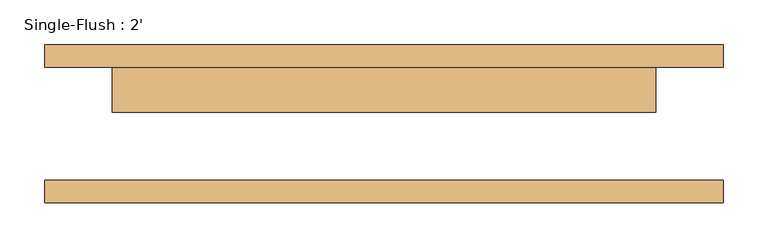
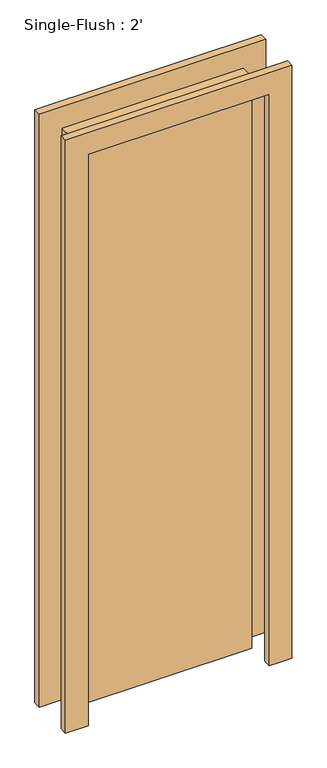
"""IFC4 building model written with IfcOpenShell, lengths in millimetres: door geometry, Single-Flush : 2'."""

from ifc_helpers import new_model, si_unit, frame, origin, origin_with_axes, place, context, project, spatial, polyline, outline, extrude, source, transform, mapped, element, save


def single_flush_2_025d1c86(model_context):
    return source(origin(), model_context, "Body", "SweptSolid", [
        extrude(outline(polyline([(2108.2, -381.0), (0.0, -381.0), (0.0, -304.8), (2032.0, -304.8), (2032.0, 304.8), (0.0, 304.8), (0.0, 381.0), (2108.2, 381.0), (2108.2, -381.0)])), frame((0.0, 63.5, 0.0), z_axis=(0.0, 1.0, 0.0), x_axis=(0.0, 0.0, 1.0)), (0.0, 0.0, 1.0), 25.4),
        extrude(outline(polyline([(2108.2, 381.0), (2108.2, -381.0), (0.0, -381.0), (0.0, -304.8), (2032.0, -304.8), (2032.0, 304.8), (0.0, 304.8), (0.0, 381.0), (2108.2, 381.0)])), frame((0.0, -88.9, 0.0), z_axis=(0.0, 1.0, 0.0), x_axis=(0.0, 0.0, 1.0)), (0.0, 0.0, 1.0), 25.4),
        extrude(outline(polyline([(304.8, 12.7), (-304.8, 12.7), (-304.8, 63.5), (304.8, 63.5), (304.8, 12.7)])), origin_with_axes(), (0.0, 0.0, 1.0), 2032.0),
    ])


if __name__ == "__main__":
    model = new_model("IFC4")
    model_context = context("Model", 3, world=origin())
    ifc_project = project(units=[si_unit("LENGTHUNIT", "METRE", prefix="MILLI")], contexts=[model_context])
    site = spatial("IfcSite", under=ifc_project)
    building = spatial("IfcBuilding", under=site)
    placement = place(None, origin())
    single_flush_2_shape = single_flush_2_025d1c86(model_context)
    element("IfcDoor", 1, ObjectType="Single-Flush : 2'", at=placement, inside=building, context=model_context, shape_type="MappedRepresentation", body=[
        mapped(single_flush_2_shape, transform((0.0, 0.0, 0.0), x_axis=(1.0, 0.0, 0.0), y_axis=(0.0, 1.0, 0.0), z_axis=(0.0, 0.0, 1.0))),
    ])
    save(model, "model.ifc")

# Revit data of these elements
# Type "Single-Flush : 2'"
#   Type Mark = "8"
#   Construction Type Id = "MDOOR"
#   Assembly Code = "C1020"
#   Analytic Construction = "Metal"
#   Thickness = 0' - 2"
#   Heat Transfer Coefficient (U) = 0.651978 BTU/(h·ft²·°F)
#   Height = 6' - 8"
#   Trim Projection Ext = 0' - 1"
#   Trim Projection Int = 0' - 1"
#   Trim Width = 0' - 3"
#   Width = 2' - 0"
#   Define Thermal Properties by = 1
#   Door Material = Door - Panel
#   Frame Material = Door - Frame
#   Visual Light Transmittance = 0
#   Solar Heat Gain Coefficient = 0
#   Function = (empty or 0)
#   Wall Closure = (empty or 0)
# Element 1 (IfcDoor, "Single-Flush : 2'")
#   Materials on its faces: "Door - Frame", "Door - Panel"
# Materials
#   "Door - Panel": class "Wood", colour RGB 210 159 95, transparency 0, Cost = 0
#   "Door - Frame": colour RGB 118 70 51, transparency 0, Cost = 0
